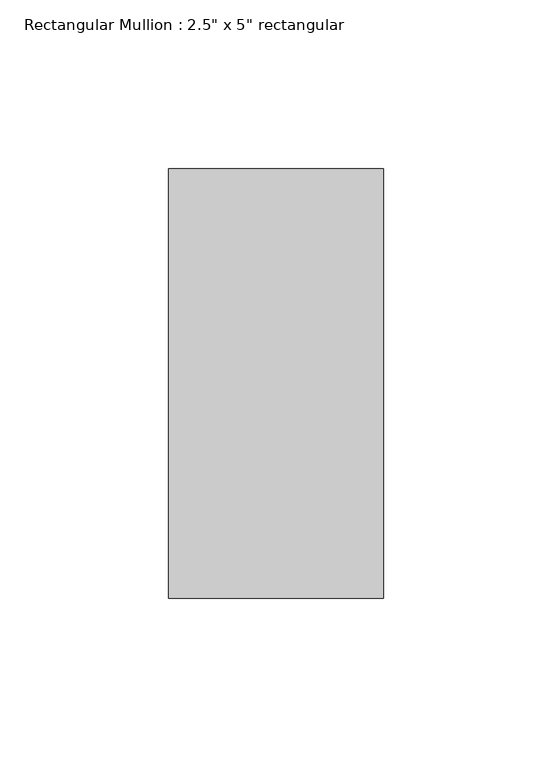
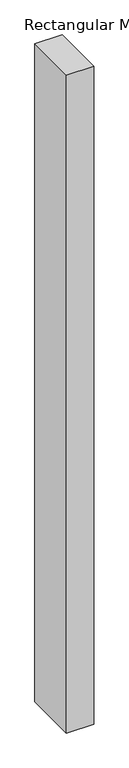
"""IFC4 building model written with IfcOpenShell, lengths in millimetres: member geometry."""

from ifc_helpers import new_model, si_unit, frame, origin, place, context, project, spatial, polyline, outline, extrude, source, transform, mapped, element, save


def member_50fd6a52(model_context):
    return source(origin(), model_context, "Body", "SweptSolid", [
        extrude(outline(polyline([(0.0, 63.5), (0.0, -63.5), (-63.5, -63.5), (-63.5, 63.5), (0.0, 63.5)])), frame((0.0, 0.0, -1616.3259354), z_axis=(0.0, 0.0, 1.0), x_axis=(1.0, 0.0, 0.0)), (0.0, 0.0, 1.0), 1616.3259354),
    ])


if __name__ == "__main__":
    model = new_model("IFC4")
    model_context = context("Model", 3, world=origin())
    ifc_project = project(units=[si_unit("LENGTHUNIT", "METRE", prefix="MILLI")], contexts=[model_context])
    site = spatial("IfcSite", under=ifc_project)
    building = spatial("IfcBuilding", under=site)
    placement = place(None, origin())
    member_shape = member_50fd6a52(model_context)
    element("IfcMember", 1, ObjectType="Rectangular Mullion : 2.5\" x 5\" rectangular", at=placement, inside=building, context=model_context, shape_type="MappedRepresentation", body=[
        mapped(member_shape, transform((0.0, 0.0, 0.0), x_axis=(1.0, 0.0, 0.0), y_axis=(0.0, 1.0, 0.0), z_axis=(0.0, 0.0, 1.0))),
    ])
    save(model, "model.ifc")

# Revit data of these elements
# Type "Rectangular Mullion : 2.5\" x 5\" rectangular"
#   built-in parameter 1007304 = 0.416667 (stored number, unit not read)
#   built-in parameter 1007301 = 0.104167 (stored number, unit not read)
#   built-in parameter 1007300 = 0.104167 (stored number, unit not read)
# Element 1 (IfcMember, "Rectangular Mullion : 2.5\" x 5\" rectangular")
#   Materials on its faces: "Aluminum"
# Materials
#   "Aluminum": class "Metal", colour RGB 247 247 247, transparency 0, Description = "Aluminum 6061", Cost = 0
